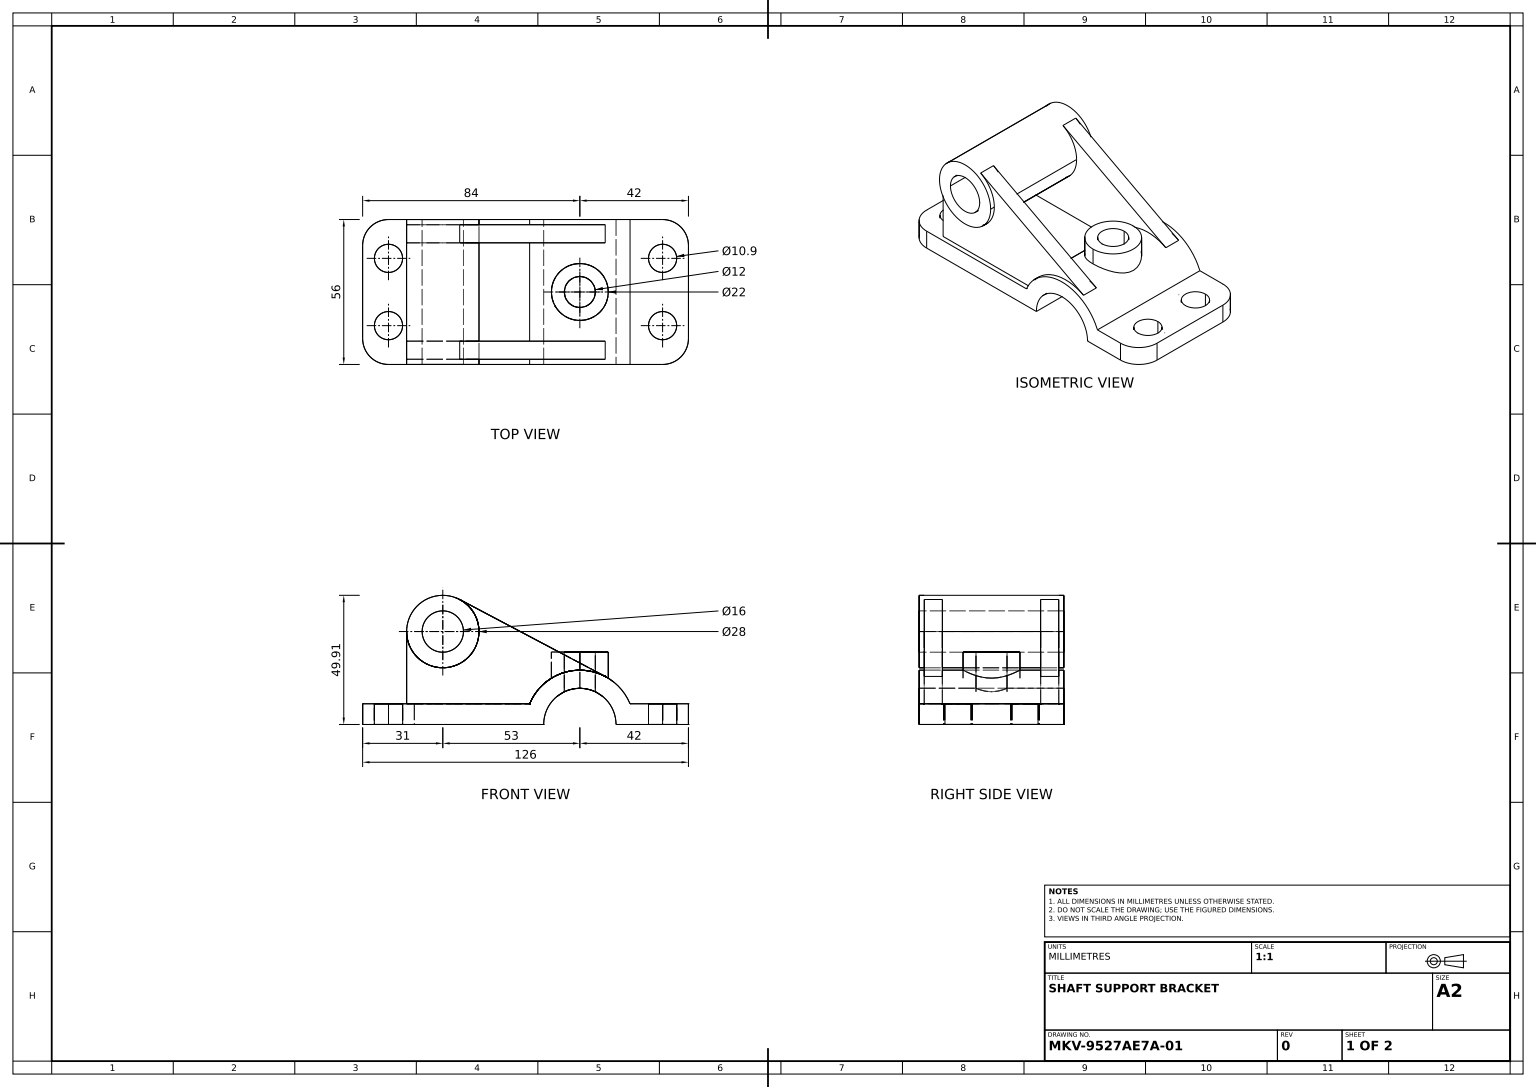
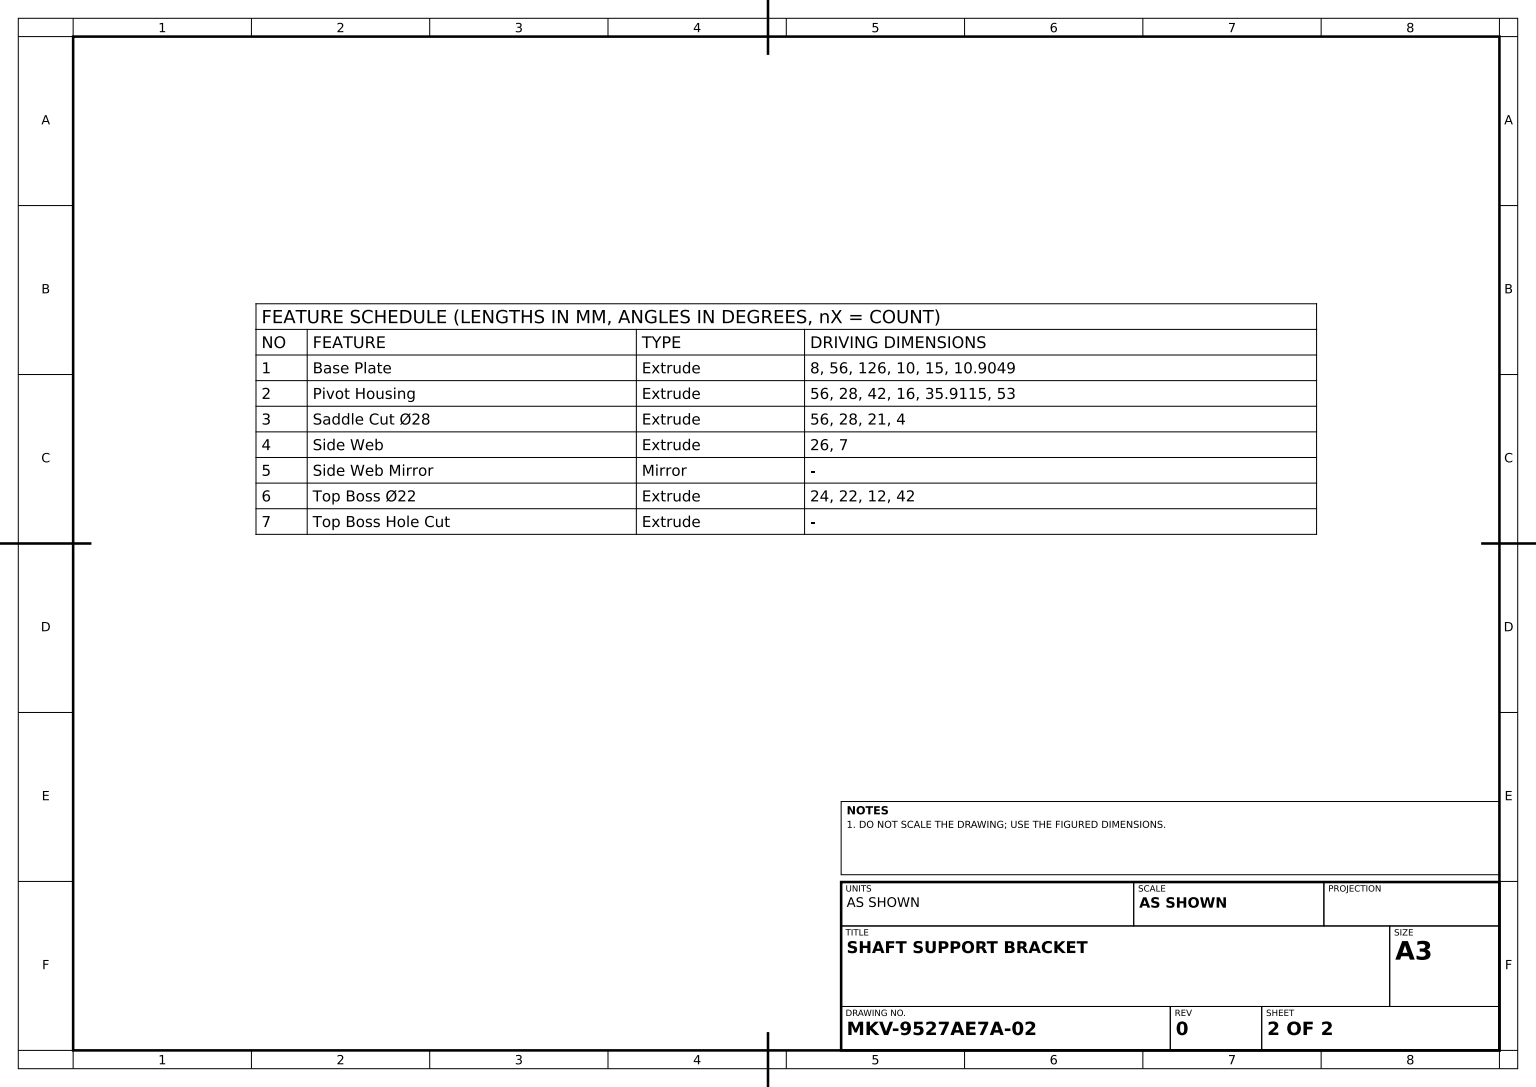
SolidWorks part; units mm, degrees
material "Plain Carbon Steel"
ref_plane "Front Plane" through (0, 0, 0) normal (0, 0, 1) x (1, 0, 0)
ref_plane "Top Plane" through (0, 0, 0) normal (0, 1, 0) x (1, 0, 0)
ref_plane "Right Plane" through (0, 0, 0) normal (1, 0, 0) x (0, 0, -1)
sketch "Base Plate Sketch" plane through (0, 0, 0) normal (0, 1, 0) x (1, 0, 0)
  line L0 (-119.533, 0) -> (130.5046, 0) construction
  line L1 (0, 101.181) -> (0, -92.4) construction
  line L3 (-53, 28) -> (53, 28)
  line L4 (-63, 18) -> (-63, -18)
  line L5 (-53, -28) -> (53, -28)
  line L6 (63, 18) -> (63, -18)
  line L7 (-63, 28) -> (63, -28) construction
  line L8 (-63, -28) -> (63, 28) construction
  arc A0 (63, -18) -> (53, -28) centre (53, -18) cw
  arc A1 (63, 18) -> (53, 28) centre (53, 18) ccw
  arc A2 (-53, -28) -> (-63, -18) centre (-53, -18) cw
  arc A3 (-63, 18) -> (-53, 28) centre (-53, 18) cw
  circle A4 centre (-53, 13) radius 5.4525
  circle A5 centre (-53, -13) radius 5.4525
  circle A6 centre (53, -13) radius 5.4525
  circle A7 centre (53, 13) radius 5.4525
  point P5 (0, 0)
  dimension "D3" = 10
  dimension "D6" = 10.9049
  dimension "D1" = 56
  dimension "D2" = 126
  dimension "D4" = 10
  dimension "D5" = 15
extrude "Base Plate" add sketch "Base Plate Sketch" along normal mid plane 8
sketch "Pivot Housing Sketch" plane through (0, 0, 0) normal (0, 0, 1) x (1, 0, 0)
  line L0 (-53, -4) -> (53, -4) construction
  line L1 (0, -4) -> (7, -4)
  line L2 (35, -4) -> (42, -4)
  line L3 (0, 35.9514) -> (0, -31.7384) construction
  arc A0 (35, -4) -> (7, -4) centre (21, -4) ccw
  arc A1 (42, -4) -> (0, -4) centre (21, -4) ccw
  circle A2 centre (-32, 31.9115) radius 14
  circle A3 centre (-32, 31.9115) radius 8
  dimension "D1" = 28
  dimension "D3" = 42
  dimension "D4" = 28
  dimension "D5" = 16
  dimension "D2" = 42
  dimension "D6" = 35.9115
  dimension "D7" = 53
extrude "Pivot Housing" add sketch "Pivot Housing Sketch" along normal mid plane 56
sketch "Saddle Cut Sketch" plane through (0, 0, 0) normal (0, 0, 1) x (1, 0, 0)
  circle A0 centre (21, -4) radius 14
  dimension "D2" = 28
  dimension "D1" = 21
  dimension "D3" = 4
extrude "Saddle Cut Ø28" cut sketch "Saddle Cut Sketch" against normal mid plane 56
ref_plane "Side Web Plane" through (0, 0, 26) normal (0, 0, 1) x (1, 0, 0)
sketch "Side Web Sketch" plane through (0, 0, 26) normal (0, 0, 1) x (1, 0, 0)
  line L0 (-53, 4) -> (1.5835, 4) construction
  line L1 (-46, 4) -> (1.5835, 4)
  line L2 (-46, 31.9115) -> (-46, 4)
  line L3 (-25.4612, 44.2907) -> (30.8082, 14.5688)
  circle A0 centre (-32, 31.9115) radius 14 construction
  arc A1 (-25.4612, 44.2907) -> (-46, 31.9115) centre (-32, 31.9115) ccw
  circle A2 centre (-32, 31.9115) radius 8 construction
  circle A3 centre (-32, 31.9115) radius 8
  arc A4 (40.4165, 4) -> (1.5835, 4) centre (21, -4) ccw construction
  arc A5 (30.8082, 14.5688) -> (1.5835, 4) centre (21, -4) ccw
extrude "Side Web" add sketch "Side Web Sketch" against normal blind 7
mirror "Side Web Mirror" about plane through (0, 0, 0) normal (0, 0, 1) of "Side Web"
ref_plane "Top Boss Plane" through (0, 24, 0) normal (0, 1, 0) x (1, 0, 0)
sketch "Top Boss Sketch" plane through (0, 24, 0) normal (0, 1, 0) x (1, 0, 0)
  line L0 (63, -18) -> (63, 18) construction
  circle A0 centre (21, 0) radius 11
  circle A1 centre (21, 0) radius 6
  dimension "D1" = 22
  dimension "D2" = 12
  dimension "D3" = 42
extrude "Top Boss Ø22" add sketch "Top Boss Sketch" against normal up to next
sketch "Top Boss Hole Sketch" plane through (0, 24, 0) normal (0, 1, 0) x (1, 0, 0)
  circle A0 centre (21, 0) radius 6 construction
  circle A1 centre (21, 0) radius 6
extrude "Top Boss Hole Cut" cut sketch "Top Boss Hole Sketch" against normal up to next
